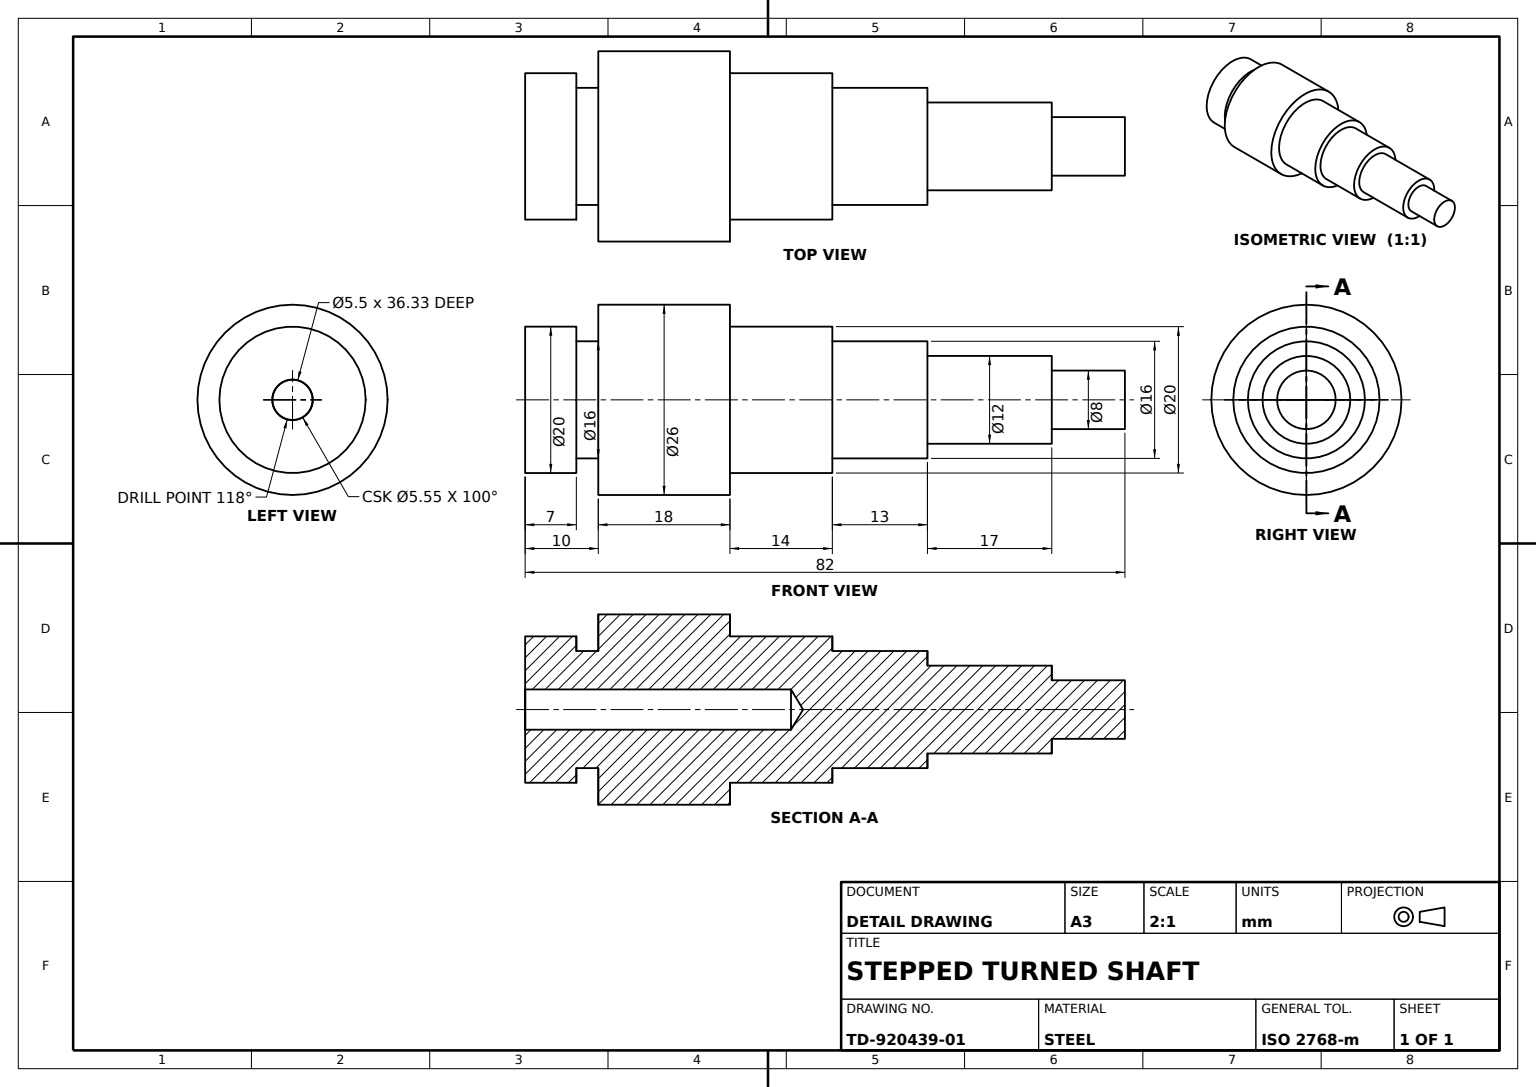
SolidWorks part; units mm, degrees
material "Plain Carbon Steel"
ref_plane "Front Plane" through (0, 0, 0) normal (0, 0, 1) x (1, 0, 0)
ref_plane "Top Plane" through (0, 0, 0) normal (0, 1, 0) x (1, 0, 0)
ref_plane "Right Plane" through (0, 0, 0) normal (1, 0, 0) x (0, 0, -1)
sketch "Shaft Profile Sketch" plane through (0, 0, 0) normal (0, 0, 1) x (1, 0, 0)
  line L0 (-602.7926, 0) -> (29537.2102, 0) construction
  line L1 (0, 0) -> (0, 10)
  line L2 (0, 10) -> (7, 10)
  line L3 (7, 10) -> (7, 8)
  line L4 (7, 8) -> (10, 8)
  line L5 (10, 8) -> (10, 13)
  line L6 (10, 13) -> (28, 13)
  line L7 (28, 13) -> (28, 10)
  line L8 (28, 10) -> (42, 10)
  line L12 (42, 10) -> (42, 8)
  line L13 (42, 8) -> (55, 8)
  line L14 (55, 8) -> (55, 6)
  line L15 (55, 6) -> (72, 6)
  line L16 (72, 6) -> (72, 4)
  line L17 (72, 4) -> (82, 4)
  line L18 (82, 4) -> (82, 0)
  line L19 (82, 0) -> (0, 0)
  dimension "D1" = 82
  dimension "D2" = 72
  dimension "D3" = 55
  dimension "D4" = 42
  dimension "D5" = 28
  dimension "D6" = 10
  dimension "D7" = 7
  dimension "D8" = 20
  dimension "D9" = 8
  dimension "D10" = 12
  dimension "D11" = 20
  dimension "D12" = 16
  dimension "D13" = 26
  dimension "D14" = 16
revolve "Stepped Shaft Revolve" add sketch "Shaft Profile Sketch" angle 360 about L0
hole_wizard "Axial Hole M5 Clearance" positions "3DSketch5" profile "Sketch6" hole size "M5" standard "ANSI Metric"
sketch3d "3DSketch5"
  point P0 (0, 0, 0)
  point P3 (0, 0, 0)
sketch "Sketch6" plane through (0, 0, 0) normal (0, 1, 0) x (0, 0, 1)
  line L0 (0, 0) -> (0, 38)
  line L1 (0, 38) -> (2.75, 36.3476)
  line L2 (2.75, 36.3476) -> (2.75, 0.021)
  line L3 (2.75, 0.021) -> (2.775, 0)
  line L5 (2.775, 0) -> (0, 0)
  line L6 (-2.75, 0.021) -> (-2.775, 0) construction
  line L10 (0, 38) -> (-2.75, 36.3476) construction
  line L11 (0, -6.35) -> (0, 107.95) construction
  dimension "Hole Dia." = 5.5
  dimension "Hole Depth" = 38
  dimension "Near C'Sink Dia." = 5.55
  dimension "Near C'Sink Angle" = 100
  dimension "Drill Angle" = 118
